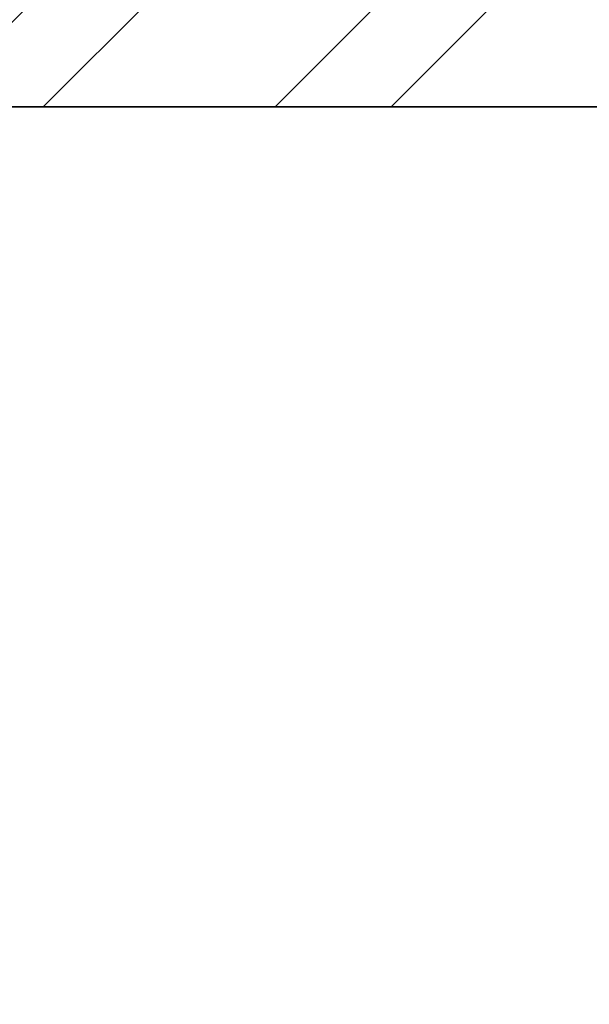
# Model space of a CAD drawing. Units: inches. Extents: x 1962 to 2771, y 1245 to 2660.
# Tile 29 of 114: x 2094 to 2116, y 1894 to 1932. Entities that reach past the tile are written whole.
import ezdxf

# ---------------------------------------------------------------- set-up
doc = ezdxf.new("R2010")
doc.units = ezdxf.units.IN
doc.layers.add('A-WALL', color=7, linetype='Continuous', lineweight=35)
doc.layers.add('A-WALL-PATT', color=252, linetype='Continuous', lineweight=13)

msp = doc.modelspace()

# ---------------------------------------------------------------- hatches: boundary and pattern name
at = {"layer": 'A-WALL-PATT'}
h = msp.add_hatch(dxfattribs=at)
h.set_pattern_fill('ANSI32', color=256)
h.paths.add_polyline_path([(2090.8074, 2467.3437), (2141.6481, 2467.3437), (2141.6481, 2469.5937), (2141.6481, 2471.8437), (2086.3074, 2471.8437), (2086.3074, 2422.5333), (2090.8074, 2422.5333)])
h.paths.add_polyline_path([(2282.7664, 2471.8437), (2204.8982, 2471.8437), (2204.8982, 2467.3437), (2234.8074, 2467.3437), (2234.8074, 2311.3437), (2228.7492, 2311.3437), (2228.7492, 2306.8437), (2234.8074, 2306.8437), (2331.9227, 2306.8437), (2331.9227, 2309.0937), (2331.9227, 2311.3437), (2239.3074, 2311.3437), (2239.3074, 2467.3437), (2282.7664, 2467.3437), (2282.7664, 2469.5937)])
h.paths.add_polyline_path([(2471.4531, 2519.8437), (2552.011, 2519.8437), (2564.3996, 2519.8437), (2564.3996, 2511.1389), (2568.8996, 2511.1389), (2568.8996, 2524.3437), (2466.9531, 2524.3437), (2466.9531, 2471.8437), (2450.0749, 2471.8437), (2446.4672, 2471.8437), (2446.4672, 2467.3437), (2450.0749, 2467.3437), (2475.9988, 2467.3437), (2475.9988, 2469.5937), (2475.9988, 2471.8437), (2471.4531, 2471.8437)])
h.paths.add_polyline_path([(2575.2231, 2469.5937), (2575.2231, 2471.8437), (2568.8996, 2471.8437), (2568.8996, 2487.1389), (2564.3996, 2487.1389), (2564.3996, 2471.8437), (2556.511, 2471.8437), (2499.2904, 2471.8437), (2499.2904, 2467.3437), (2507.8074, 2467.3437), (2507.8074, 2311.3437), (2414.863, 2311.3437), (2414.863, 2306.8437), (2512.3074, 2306.8437), (2517.0114, 2306.8437), (2517.0114, 2309.0937), (2517.0114, 2311.3437), (2512.3074, 2311.3437), (2512.3074, 2467.3437), (2575.2231, 2467.3437)])
h.paths.add_polyline_path([(2660.8074, 2471.8437), (2600.9602, 2471.8437), (2600.9602, 2467.3437), (2656.3074, 2467.3437), (2656.3074, 2432.5704), (2660.8074, 2432.5704)])
h.paths.add_polyline_path([(2660.8074, 2372.5704), (2656.3074, 2372.5704), (2656.3074, 2311.3437), (2600.276, 2311.3437), (2600.276, 2309.0937), (2600.276, 2306.8437), (2656.3074, 2306.8437), (2656.3074, 2296.2593), (2660.8074, 2296.2593)])
h.paths.add_polyline_path([(2572.3074, 2306.8437), (2577.1385, 2306.8437), (2577.1385, 2311.3437), (2551.082, 2311.3437), (2551.082, 2306.8437), (2567.8074, 2306.8437), (2567.8074, 2258.8437), (2540.0574, 2258.8437), (2540.0574, 2256.5937), (2540.0574, 2254.3437), (2567.8074, 2254.3437), (2656.3074, 2254.3437), (2656.3074, 2236.9085), (2660.8074, 2236.9085), (2660.8074, 2272.2593), (2656.3074, 2272.2593), (2656.3074, 2258.8437), (2572.3074, 2258.8437)])
h.paths.add_polyline_path([(2512.3074, 2254.3437), (2518.8716, 2254.3437), (2518.8716, 2256.5937), (2518.8716, 2258.8437), (2507.8074, 2258.8437), (2507.8074, 2177.8437), (2567.8074, 2177.8437), (2567.8074, 2172.9628), (2572.3074, 2172.9628), (2572.3074, 2177.8437), (2656.3074, 2177.8437), (2656.3074, 2166.4846), (2660.8074, 2166.4846), (2660.8074, 2200.9085), (2656.3074, 2200.9085), (2656.3074, 2182.3437), (2512.3074, 2182.3437)])
h.paths.add_polyline_path([(2656.3074, 2129.8437), (2572.3074, 2129.8437), (2572.3074, 2150.3044), (2570.0574, 2150.3044), (2567.8074, 2150.3044), (2567.8074, 2129.8437), (2507.8074, 2129.8437), (2507.8074, 2116.3027), (2510.0574, 2116.3027), (2512.3074, 2116.3027), (2512.3074, 2125.3437), (2567.8074, 2125.3437), (2572.3074, 2125.3437), (2656.3074, 2125.3437)])
h.paths.add_polyline_path([(2090.8074, 2362.5333), (2086.3074, 2362.5333), (2086.3074, 2298.6242), (2090.8074, 2298.6242), (2090.8074, 2306.8437), (2174.8074, 2306.8437), (2174.8074, 2286.4178), (2179.3074, 2286.4178), (2179.3074, 2306.8437), (2192.8641, 2306.8437), (2192.8641, 2309.0937), (2192.8641, 2311.3437), (2090.8074, 2311.3437)])
h.paths.add_polyline_path([(2209.156, 2258.8437), (2179.3074, 2258.8437), (2179.3074, 2263.2236), (2177.0574, 2263.2236), (2174.8074, 2263.2236), (2174.8074, 2258.8437), (2090.8074, 2258.8437), (2090.8074, 2274.6242), (2086.3074, 2274.6242), (2086.3074, 2238.2967), (2088.5574, 2238.2967), (2090.8074, 2238.2967), (2090.8074, 2254.3437), (2209.156, 2254.3437)])
h.paths.add_polyline_path([(2090.8074, 2177.8437), (2234.8074, 2177.8437), (2234.8074, 2173.1428), (2239.3074, 2173.1428), (2239.3074, 2258.8437), (2230.8442, 2258.8437), (2230.8442, 2256.5937), (2230.8442, 2254.3437), (2234.8074, 2254.3437), (2234.8074, 2182.3437), (2090.8074, 2182.3437), (2090.8074, 2202.2967), (2086.3074, 2202.2967), (2086.3074, 2140.0389), (2090.8074, 2140.0389)])
h.paths.add_polyline_path([(2090.8074, 2080.0389), (2086.3074, 2080.0389), (2086.3074, 2033.8437), (2090.8074, 2033.8437)], flags=17)
h.paths.add_polyline_path([(2244.9405, 2033.8437), (2239.3074, 2033.8437), (2239.3074, 2142.0665), (2237.2592, 2142.0665), (2234.8074, 2142.0665), (2234.8074, 2033.8437), (2090.8074, 2033.8437), (2076.5204, 2033.8437), (2072.0204, 2033.8437), (2072.0204, 2000.4493), (2076.5204, 2000.4493), (2076.5204, 2029.3437), (2090.8074, 2029.3437), (2244.9405, 2029.3437), (2244.9405, 2031.5937)])
h.paths.add_polyline_path([(2234.8074, 1933.3437), (2076.5204, 1933.3437), (2076.5204, 1952.4493), (2074.2704, 1952.4493), (2072.0204, 1952.4493), (2072.0204, 1933.3437), (2072.0204, 1928.8437), (2234.8074, 1928.8437)])
h.paths.add_polyline_path([(2090.8074, 1928.8437), (2086.3074, 1928.8437), (2086.3074, 1906.5013), (2090.8074, 1906.5013)])
h.paths.add_polyline_path([(2090.8074, 1846.5013), (2086.3074, 1846.5013), (2086.3074, 1769.9917), (2088.5574, 1769.9917), (2090.8074, 1769.9917), (2090.8074, 1780.3437), (2234.8074, 1780.3437), (2234.8074, 1708.3437), (2230.3764, 1708.3437), (2230.3764, 1703.8437), (2239.3074, 1703.8437), (2239.3074, 1792.6669), (2237.0574, 1792.6669), (2234.8074, 1792.6669), (2234.8074, 1784.8437), (2090.8074, 1784.8437)])
h.paths.add_polyline_path([(2239.3074, 1928.8437), (2244.9405, 1928.8437), (2244.9405, 1931.0937), (2244.9405, 1933.3437), (2234.8074, 1933.3437), (2234.8074, 1928.8437), (2234.8074, 1825.5949), (2239.3074, 1825.5949)])
h.paths.add_polyline_path([(2148.0425, 1649.0937), (2148.0425, 1651.3437), (2090.8074, 1651.3437), (2090.8074, 1646.8437), (2148.0425, 1646.8437)], flags=0)
h.paths.add_polyline_path([(2207.5601, 1708.3437), (2090.8074, 1708.3437), (2090.8074, 1703.8437), (2174.8074, 1703.8437), (2174.8074, 1651.3437), (2170.4457, 1651.3437), (2170.4457, 1646.8437), (2195.9924, 1646.8437), (2195.9924, 1649.0937), (2195.9924, 1651.3437), (2179.3074, 1651.3437), (2179.3074, 1703.8437), (2207.5601, 1703.8437), (2207.5601, 1706.0937)])
h.paths.add_polyline_path([(2090.8074, 1733.9917), (2086.3074, 1733.9917), (2086.3074, 1696.1032), (2088.5574, 1696.1032), (2090.8074, 1696.1032)])
h.paths.add_polyline_path([(2090.8074, 1672.1032), (2086.3074, 1672.1032), (2086.3074, 1600.3335), (2090.8074, 1600.3335)])
h.paths.add_polyline_path([(2090.8074, 1540.3335), (2086.3074, 1540.3335), (2086.3074, 1486.3437), (2139.6766, 1486.3437), (2139.6766, 1490.8437), (2090.8074, 1490.8437)])
h.paths.add_polyline_path([(2302.3876, 1490.8437), (2239.3074, 1490.8437), (2239.3074, 1646.8437), (2335.9994, 1646.8437), (2335.9994, 1651.3437), (2229.884, 1651.3437), (2229.884, 1646.8437), (2234.8074, 1646.8437), (2234.8074, 1490.8437), (2202.7103, 1490.8437), (2202.7103, 1488.5937), (2202.7103, 1486.3437), (2275.0699, 1486.3437), (2275.0699, 1475.772), (2279.5699, 1475.772), (2279.5699, 1486.3437), (2302.3876, 1486.3437)])
h.paths.add_polyline_path([(2279.5699, 1451.772), (2275.0699, 1451.772), (2275.0699, 1438.3437), (2174.8074, 1438.3437), (2174.8074, 1486.3437), (2179.7922, 1486.3437), (2179.7922, 1490.8437), (2163.3585, 1490.8437), (2163.3585, 1488.5937), (2163.3585, 1486.3437), (2170.3074, 1486.3437), (2170.3074, 1433.8437), (2279.5699, 1433.8437)])
h.paths.add_polyline_path([(2427.2363, 1490.8437), (2375.8074, 1490.8437), (2375.8074, 1646.8437), (2381.6401, 1646.8437), (2381.6401, 1651.3437), (2365.887, 1651.3437), (2365.887, 1649.0937), (2365.887, 1646.8437), (2371.3074, 1646.8437), (2371.3074, 1490.8437), (2327.5627, 1490.8437), (2327.5627, 1488.5937), (2327.5627, 1486.3437), (2371.3074, 1486.3437), (2371.3074, 1433.8437), (2375.8074, 1433.8437), (2375.8074, 1486.3437), (2427.2363, 1486.3437)])
h.paths.add_polyline_path([(2512.3074, 1646.8437), (2519.4351, 1646.8437), (2519.4351, 1649.0937), (2519.4351, 1651.3437), (2507.8074, 1651.3437), (2416.0063, 1651.3437), (2416.0063, 1649.0937), (2416.0063, 1646.8437), (2507.8074, 1646.8437), (2507.8074, 1490.8437), (2497.0532, 1490.8437), (2497.0532, 1488.5937), (2497.0532, 1486.3437), (2574.9344, 1486.3437), (2574.9344, 1476.0181), (2579.4344, 1476.0181), (2579.4344, 1486.3437), (2584.4872, 1486.3437), (2584.3074, 1490.8437), (2512.3074, 1490.8437)])
h.paths.add_polyline_path([(2470.5091, 1486.3437), (2473.9767, 1486.3437), (2473.9767, 1490.8437), (2449.6605, 1490.8437), (2449.6605, 1488.5937), (2449.6605, 1486.3437), (2466.0091, 1486.3437), (2466.0091, 1433.8437), (2470.5091, 1433.8437), (2579.4344, 1433.8437), (2579.4344, 1452.0181), (2574.9344, 1452.0181), (2574.9344, 1438.3437), (2554.5091, 1438.3437), (2470.5091, 1438.3437)])
h.paths.add_polyline_path([(2656.3074, 1490.8437), (2611.86, 1490.8437), (2611.86, 1486.3437), (2656.3074, 1486.3437)])
h.paths.add_polyline_path([(2660.8074, 1532.7007), (2658.5574, 1532.7007), (2656.3074, 1532.7007), (2656.3074, 1486.3437), (2660.8074, 1486.3437)])
h.paths.add_polyline_path([(2660.8074, 1664.9663), (2656.3074, 1664.9663), (2656.3074, 1651.3437), (2602.2313, 1651.3437), (2602.2313, 1646.8437), (2656.3074, 1646.8437), (2656.3074, 1592.7007), (2660.8074, 1592.7007)])
h.paths.add_polyline_path([(2660.8074, 1724.5221), (2656.3074, 1724.5221), (2656.3074, 1703.8437), (2542.4725, 1703.8437), (2542.4725, 1699.3437), (2567.8074, 1699.3437), (2567.8074, 1651.3437), (2552.7766, 1651.3437), (2552.7766, 1649.0937), (2552.7766, 1646.8437), (2577.2878, 1646.8437), (2577.2878, 1649.0937), (2577.2878, 1651.3437), (2572.3074, 1651.3437), (2572.3074, 1699.3437), (2656.3074, 1699.3437), (2656.3074, 1688.9663), (2660.8074, 1688.9663)])
h.paths.add_polyline_path([(2660.8074, 1880.6524), (2656.3074, 1880.6524), (2656.3074, 1832.8437), (2512.3074, 1832.8437), (2512.3074, 1837.8959), (2507.8074, 1837.8959), (2507.8074, 1828.3437), (2567.8074, 1828.3437), (2567.8074, 1804.3437), (2572.3074, 1804.3437), (2572.3074, 1828.3437), (2656.3074, 1828.3437), (2656.3074, 1818.6778), (2660.8074, 1818.6778)])
h.paths.add_polyline_path([(2660.8074, 1794.6778), (2656.3074, 1794.6778), (2656.3074, 1780.3437), (2572.3074, 1780.3437), (2572.3074, 1783.0303), (2570.0574, 1783.0303), (2567.8074, 1783.0303), (2567.8074, 1780.3437), (2507.8074, 1780.3437), (2507.8074, 1699.3437), (2517.8858, 1699.3437), (2517.8858, 1701.5937), (2517.8858, 1703.8437), (2512.3074, 1703.8437), (2512.3074, 1775.8437), (2656.3074, 1775.8437), (2656.3074, 1760.5221), (2660.8074, 1760.5221)])
h.paths.add_polyline_path([(2660.8074, 1981.3437), (2660.8074, 2020.2808), (2658.5574, 2020.2808), (2656.3074, 2020.2808), (2656.3074, 1981.3437), (2512.3074, 1981.3437), (2512.3074, 2086.6996), (2507.8074, 2086.6996), (2507.8074, 1981.3437), (2375.8074, 1981.3437), (2375.8074, 1986.8505), (2373.5574, 1986.8505), (2371.3074, 1986.8505), (2371.3074, 1973.2607), (2375.8074, 1973.2607), (2375.8074, 1976.8437), (2507.8074, 1976.8437), (2507.8074, 1865.4281), (2510.0574, 1865.4281), (2512.3074, 1865.4281), (2512.3074, 1976.8437), (2660.8074, 1976.8437)])
h.paths.add_polyline_path([(2375.8074, 1940.297), (2373.5574, 1940.297), (2371.3074, 1940.297), (2371.3074, 1933.3437), (2278.4434, 1933.3437), (2278.4434, 1928.8437), (2371.3074, 1928.8437), (2371.3074, 1651.3437), (2375.8074, 1651.3437)])
h.paths.add_polyline_path([(2660.8074, 1976.8437), (2656.3074, 1976.8437), (2656.3074, 1940.6524), (2660.8074, 1940.6524)], flags=17)
h.paths.add_polyline_path([(2660.8074, 2142.4846), (2656.3074, 2142.4846), (2656.3074, 2080.2808), (2660.8074, 2080.2808)])
h.paths.add_polyline_path([(2381.4189, 2311.3437), (2375.8074, 2311.3437), (2375.8074, 2467.3437), (2424.7242, 2467.3437), (2424.7242, 2469.5937), (2424.7242, 2471.8437), (2375.8074, 2471.8437), (2375.8074, 2524.3437), (2371.3074, 2524.3437), (2371.3074, 2471.8437), (2307.2097, 2471.8437), (2307.2097, 2467.3437), (2371.3074, 2467.3437), (2371.3074, 2311.3437), (2366.8901, 2311.3437), (2366.8901, 2306.8437), (2371.3074, 2306.8437), (2371.3074, 2033.8437), (2279.6589, 2033.8437), (2279.6589, 2029.3437), (2371.3074, 2029.3437), (2371.3074, 2014.2598), (2375.8074, 2014.2598), (2375.8074, 2306.8437), (2381.4189, 2306.8437)])
h.paths.add_polyline_path([(2263.3074, 2524.3437), (2170.3074, 2524.3437), (2170.3074, 2519.8437), (2170.3074, 2471.8437), (2165.0312, 2471.8437), (2165.0312, 2467.3437), (2179.6721, 2467.3437), (2179.6721, 2469.5161), (2179.6721, 2471.8437), (2174.8074, 2471.8437), (2174.8074, 2519.8437), (2258.8074, 2519.8437), (2258.8074, 2511.6436), (2263.3074, 2511.6436)])
h.paths.add_polyline_path([(2245.0232, 1361.4123), (2492.9468, 1361.4123), (2492.9468, 1398.505), (2245.0232, 1398.505)], flags=9)
h.paths.add_polyline_path([(2388.1434, 2086.6936), (2425.0704, 2086.6936), (2425.0704, 2105.3509), (2388.1434, 2105.3509)], flags=9)
h.paths.add_polyline_path([(2404.922, 2242.6744), (2445.7337, 2242.6744), (2445.7337, 2261.3318), (2404.922, 2261.3318)], flags=9)
h.paths.add_polyline_path([(2269.4107, 2156.7935), (2306.3378, 2156.7935), (2306.3378, 2175.4508), (2269.4107, 2175.4508)], flags=9)
h.paths.add_polyline_path([(2269.3277, 2233.4343), (2306.2547, 2233.4343), (2306.2547, 2252.0917), (2269.3277, 2252.0917)], flags=9)
h.paths.add_polyline_path([(2431.6052, 2320.6922), (2470.4456, 2320.6922), (2470.4456, 2339.3495), (2431.6052, 2339.3495)], flags=25)
h.paths.add_polyline_path([(2249.6902, 2315.7608), (2288.5306, 2315.7608), (2288.5306, 2334.4182), (2249.6902, 2334.4182)], flags=25)
h.paths.add_polyline_path([(2096.9301, 2314.3181), (2135.7704, 2314.3181), (2135.7704, 2332.9755), (2096.9301, 2332.9755)], flags=25)
h.paths.add_polyline_path([(2134.3475, 2285.7089), (2161.4655, 2285.7089), (2161.4655, 2304.3662), (2134.3475, 2304.3662)], flags=9)
h.paths.add_polyline_path([(2126.5155, 2209.4076), (2159.9227, 2209.4076), (2159.9227, 2228.065), (2126.5155, 2228.065)], flags=25)
h.paths.add_polyline_path([(2110.5753, 2141.5299), (2149.4157, 2141.5299), (2149.4157, 2160.1872), (2110.5753, 2160.1872)], flags=25)
h.paths.add_polyline_path([(2249.8618, 1968.3317), (2286.3966, 1968.3317), (2286.3966, 1986.989), (2249.8618, 1986.989)], flags=9)
h.paths.add_polyline_path([(2395.9507, 1777.0051), (2436.7624, 1777.0051), (2436.7624, 1795.6625), (2395.9507, 1795.6625)], flags=9)
h.paths.add_polyline_path([(2398.5259, 1888.5651), (2435.0062, 1888.5651), (2435.0062, 1907.2224), (2398.5259, 1907.2224)], flags=25)
h.paths.add_polyline_path([(2259.3506, 1728.3559), (2296.2776, 1728.3559), (2296.2776, 1747.0132), (2259.3506, 1747.0132)], flags=9)
h.paths.add_polyline_path([(2271.3698, 1845.268), (2308.2968, 1845.268), (2308.2968, 1863.9253), (2271.3698, 1863.9253)], flags=9)
h.paths.add_polyline_path([(2120.9355, 1786.3027), (2159.7759, 1786.3027), (2159.7759, 1804.9601), (2120.9355, 1804.9601)], flags=25)
h.paths.add_polyline_path([(2121.3164, 1732.1043), (2154.7236, 1732.1043), (2154.7236, 1750.7616), (2121.3164, 1750.7616)], flags=25)
h.paths.add_polyline_path([(2118.3706, 1678.8997), (2147.5282, 1678.8997), (2147.5282, 1697.557), (2118.3706, 1697.557)], flags=25)
h.paths.add_polyline_path([(2385.9227, 1493.557), (2424.763, 1493.557), (2424.763, 1512.2143), (2385.9227, 1512.2143)], flags=25)
h.paths.add_polyline_path([(2248.7058, 1500.0256), (2287.5462, 1500.0256), (2287.5462, 1518.6829), (2248.7058, 1518.6829)], flags=25)
h.paths.add_polyline_path([(2104.1669, 1617.3771), (2143.0073, 1617.3771), (2143.0073, 1636.0344), (2104.1669, 1636.0344)], flags=9)
h.paths.add_polyline_path([(2096.0714, 1447.8824), (2137.3845, 1447.8824), (2137.3845, 1458.1859), (2096.0714, 1458.1859)], flags=9)
h.paths.add_polyline_path([(2180.6114, 1440.325), (2209.7689, 1440.325), (2209.7689, 1458.9823), (2180.6114, 1458.9823)], flags=25)
h.paths.add_polyline_path([(2316.1698, 1447.9637), (2357.4829, 1447.9637), (2357.4829, 1458.2673), (2316.1698, 1458.2673)], flags=9)
h.paths.add_polyline_path([(2397.6187, 1447.9637), (2438.9318, 1447.9637), (2438.9318, 1458.2673), (2397.6187, 1458.2673)], flags=9)
h.paths.add_polyline_path([(2473.0778, 1439.5953), (2502.2354, 1439.5953), (2502.2354, 1458.2527), (2473.0778, 1458.2527)], flags=25)
h.paths.add_polyline_path([(2589.7027, 1447.8819), (2631.0158, 1447.8819), (2631.0158, 1458.1855), (2589.7027, 1458.1855)], flags=9)
h.paths.add_polyline_path([(2522.4009, 1497.5285), (2561.2413, 1497.5285), (2561.2413, 1516.1859), (2522.4009, 1516.1859)], flags=25)
h.paths.add_polyline_path([(2579.6565, 1671.3482), (2608.8141, 1671.3482), (2608.8141, 1690.0056), (2579.6565, 1690.0056)], flags=25)
h.paths.add_polyline_path([(2544.7038, 1725.5064), (2578.1111, 1725.5064), (2578.1111, 1744.1637), (2544.7038, 1744.1637)], flags=25)
h.paths.add_polyline_path([(2578.1191, 1807.472), (2607.2766, 1807.472), (2607.2766, 1826.1293), (2578.1191, 1826.1293)], flags=25)
h.paths.add_polyline_path([(2595.0614, 1835.1839), (2633.9018, 1835.1839), (2633.9018, 1853.8413), (2595.0614, 1853.8413)], flags=25)
h.paths.add_polyline_path([(2567.0097, 2097.7035), (2605.8501, 2097.7035), (2605.8501, 2116.3609), (2567.0097, 2116.3609)], flags=9)
h.paths.add_polyline_path([(2586.644, 2134.6454), (2615.8015, 2134.6454), (2615.8015, 2153.3027), (2586.644, 2153.3027)], flags=9)
h.paths.add_polyline_path([(2544.6185, 2212.6783), (2578.0258, 2212.6783), (2578.0258, 2231.3356), (2544.6185, 2231.3356)], flags=25)
h.paths.add_polyline_path([(2577.0273, 2256.9023), (2606.1849, 2256.9023), (2606.1849, 2275.5597), (2577.0273, 2275.5597)], flags=24)
h.paths.add_polyline_path([(2605.2683, 2315.2821), (2644.1087, 2315.2821), (2644.1087, 2333.9395), (2605.2683, 2333.9395)], flags=25)
h.paths.add_polyline_path([(2583.1244, 2496.1815), (2624.4375, 2496.1815), (2624.4375, 2506.4851), (2583.1244, 2506.4851)], flags=9)
h.paths.add_polyline_path([(2474.761, 2497.0823), (2503.9185, 2497.0823), (2503.9185, 2515.7397), (2474.761, 2515.7397)], flags=25)
h.paths.add_polyline_path([(2387.5787, 2494.2563), (2428.902, 2494.2563), (2428.902, 2504.5598), (2387.5787, 2504.5598)], flags=9)
h.paths.add_polyline_path([(2300.1657, 2500.1564), (2341.4788, 2500.1564), (2341.4788, 2510.46), (2300.1657, 2510.46)], flags=25)
h.paths.add_polyline_path([(2176.8589, 2497.5843), (2206.0165, 2497.5843), (2206.0165, 2516.2416), (2176.8589, 2516.2416)], flags=25)
h.paths.add_polyline_path([(2097.4668, 2494.9762), (2138.7799, 2494.9762), (2138.7799, 2505.2798), (2097.4668, 2505.2798)], flags=9)

# ---------------------------------------------------------------- linework, layer by layer
at = {"layer": 'A-WALL'}
msp.add_line((2072.0204, 1928.8437), (2234.8074, 1928.8437), dxfattribs=at)

doc.saveas('drawing.dxf')
